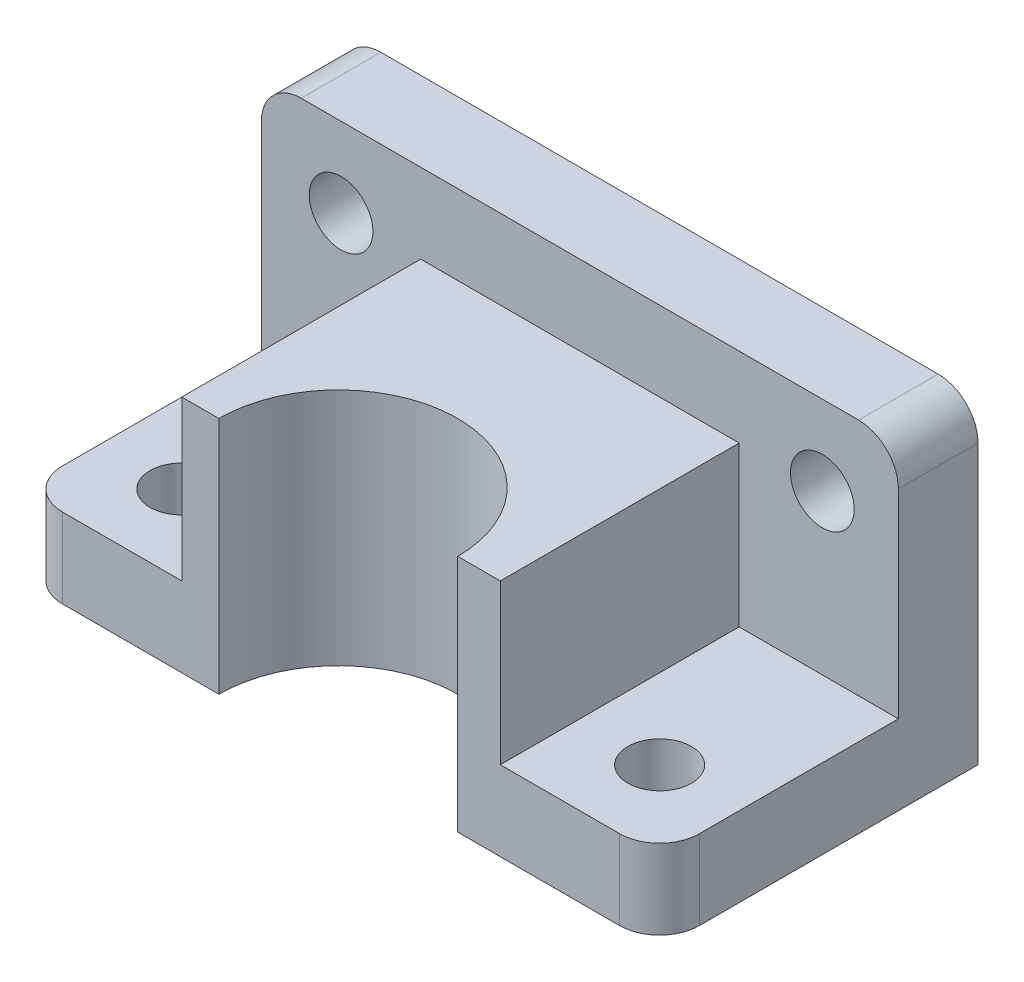
ISO-10303-21;
HEADER;
FILE_DESCRIPTION(('STEP AP214'),'2;1');
FILE_NAME('part.step','',(''),(''),'','','');
FILE_SCHEMA(('AUTOMOTIVE_DESIGN { 1 0 10303 214 1 1 1 1 }'));
ENDSEC;
DATA;
#1=APPLICATION_CONTEXT('core data for automotive mechanical design processes');
#2=APPLICATION_PROTOCOL_DEFINITION('international standard','automotive_design',2000,#1);
#3=PRODUCT_CONTEXT('',#1,'mechanical');
#4=PRODUCT('Part','Part','',(#3));
#5=PRODUCT_RELATED_PRODUCT_CATEGORY('part','',(#4));
#6=PRODUCT_DEFINITION_FORMATION('','',#4);
#7=PRODUCT_DEFINITION_CONTEXT('part definition',#1,'design');
#8=PRODUCT_DEFINITION('design','',#6,#7);
#9=PRODUCT_DEFINITION_SHAPE('','',#8);
#10=(LENGTH_UNIT() NAMED_UNIT(*) SI_UNIT(.MILLI.,.METRE.));
#11=(NAMED_UNIT(*) PLANE_ANGLE_UNIT() SI_UNIT($,.RADIAN.));
#12=(NAMED_UNIT(*) SI_UNIT($,.STERADIAN.) SOLID_ANGLE_UNIT());
#13=UNCERTAINTY_MEASURE_WITH_UNIT(LENGTH_MEASURE(1.E-05),#10,'distance_accuracy_value','');
#14=(GEOMETRIC_REPRESENTATION_CONTEXT(3) GLOBAL_UNCERTAINTY_ASSIGNED_CONTEXT((#13)) GLOBAL_UNIT_ASSIGNED_CONTEXT((#10,
#11,#12)) REPRESENTATION_CONTEXT('',''));
#15=CARTESIAN_POINT('',(0.,0.,0.));
#16=DIRECTION('',(0.,0.,1.));
#17=DIRECTION('',(1.,0.,0.));
#18=AXIS2_PLACEMENT_3D('',#15,#16,#17);
#19=CARTESIAN_POINT('',(5.,35.,10.));
#20=DIRECTION('',(0.,0.,1.));
#21=DIRECTION('',(1.,0.,0.));
#22=AXIS2_PLACEMENT_3D('',#19,#20,#21);
#23=PLANE('',#22);
#24=CARTESIAN_POINT('',(10.,30.,10.));
#25=DIRECTION('',(0.,0.,1.));
#26=DIRECTION('',(1.,0.,0.));
#27=AXIS2_PLACEMENT_3D('',#24,#25,#26);
#28=CIRCLE('',#27,4.);
#29=CARTESIAN_POINT('',(14.,30.,10.));
#30=VERTEX_POINT('',#29);
#31=EDGE_CURVE('E412',#30,#30,#28,.T.);
#32=ORIENTED_EDGE('',*,*,#31,.F.);
#33=EDGE_LOOP('',(#32));
#34=FACE_BOUND('',#33,.T.);
#35=CARTESIAN_POINT('',(70.4471624611322,30.,10.));
#36=DIRECTION('',(0.,0.,1.));
#37=DIRECTION('',(1.,0.,0.));
#38=AXIS2_PLACEMENT_3D('',#35,#36,#37);
#39=CIRCLE('',#38,3.99999999999999);
#40=CARTESIAN_POINT('',(74.4471624611322,30.,10.));
#41=VERTEX_POINT('',#40);
#42=EDGE_CURVE('E404',#41,#41,#39,.T.);
#43=ORIENTED_EDGE('',*,*,#42,.F.);
#44=EDGE_LOOP('',(#43));
#45=FACE_BOUND('',#44,.T.);
#46=DIRECTION('',(0.,-1.,0.));
#47=VECTOR('',#46,1.);
#48=CARTESIAN_POINT('',(20.,30.,10.));
#49=LINE('',#48,#47);
#50=CARTESIAN_POINT('',(20.,30.,10.));
#51=VERTEX_POINT('',#50);
#52=CARTESIAN_POINT('',(20.,10.,10.));
#53=VERTEX_POINT('',#52);
#54=EDGE_CURVE('E63',#51,#53,#49,.T.);
#55=ORIENTED_EDGE('',*,*,#54,.F.);
#56=DIRECTION('',(1.,0.,0.));
#57=VECTOR('',#56,1.);
#58=CARTESIAN_POINT('',(20.,30.,10.));
#59=LINE('',#58,#57);
#60=CARTESIAN_POINT('',(60.,30.,10.));
#61=VERTEX_POINT('',#60);
#62=EDGE_CURVE('E58',#51,#61,#59,.T.);
#63=ORIENTED_EDGE('',*,*,#62,.T.);
#64=DIRECTION('',(0.,-1.,0.));
#65=VECTOR('',#64,1.);
#66=CARTESIAN_POINT('',(60.,30.,10.));
#67=LINE('',#66,#65);
#68=CARTESIAN_POINT('',(60.,10.,10.));
#69=VERTEX_POINT('',#68);
#70=EDGE_CURVE('E171',#61,#69,#67,.T.);
#71=ORIENTED_EDGE('',*,*,#70,.T.);
#72=DIRECTION('',(1.,0.,0.));
#73=VECTOR('',#72,1.);
#74=CARTESIAN_POINT('',(60.,10.,10.));
#75=LINE('',#74,#73);
#76=CARTESIAN_POINT('',(80.,10.,10.));
#77=VERTEX_POINT('',#76);
#78=EDGE_CURVE('E206',#69,#77,#75,.T.);
#79=ORIENTED_EDGE('',*,*,#78,.T.);
#80=DIRECTION('',(0.,1.,0.));
#81=VECTOR('',#80,1.);
#82=CARTESIAN_POINT('',(80.,0.,10.));
#83=LINE('',#82,#81);
#84=CARTESIAN_POINT('',(80.,35.,10.));
#85=VERTEX_POINT('',#84);
#86=EDGE_CURVE('E259',#77,#85,#83,.T.);
#87=ORIENTED_EDGE('',*,*,#86,.T.);
#88=CARTESIAN_POINT('',(75.,35.,10.));
#89=DIRECTION('',(0.,0.,1.));
#90=DIRECTION('',(1.,0.,0.));
#91=AXIS2_PLACEMENT_3D('',#88,#89,#90);
#92=CIRCLE('',#91,5.);
#93=CARTESIAN_POINT('',(75.,40.,10.));
#94=VERTEX_POINT('',#93);
#95=EDGE_CURVE('E261',#85,#94,#92,.T.);
#96=ORIENTED_EDGE('',*,*,#95,.T.);
#97=DIRECTION('',(-1.,0.,0.));
#98=VECTOR('',#97,1.);
#99=CARTESIAN_POINT('',(5.,40.,10.));
#100=LINE('',#99,#98);
#101=CARTESIAN_POINT('',(5.,40.,10.));
#102=VERTEX_POINT('',#101);
#103=EDGE_CURVE('E263',#94,#102,#100,.T.);
#104=ORIENTED_EDGE('',*,*,#103,.T.);
#105=CARTESIAN_POINT('',(5.,35.,10.));
#106=DIRECTION('',(0.,0.,1.));
#107=DIRECTION('',(1.,0.,0.));
#108=AXIS2_PLACEMENT_3D('',#105,#106,#107);
#109=CIRCLE('',#108,5.);
#110=CARTESIAN_POINT('',(0.,35.,10.));
#111=VERTEX_POINT('',#110);
#112=EDGE_CURVE('E264',#102,#111,#109,.T.);
#113=ORIENTED_EDGE('',*,*,#112,.T.);
#114=DIRECTION('',(0.,-1.,0.));
#115=VECTOR('',#114,1.);
#116=CARTESIAN_POINT('',(0.,0.,10.));
#117=LINE('',#116,#115);
#118=CARTESIAN_POINT('',(0.,10.,10.));
#119=VERTEX_POINT('',#118);
#120=EDGE_CURVE('E253',#111,#119,#117,.T.);
#121=ORIENTED_EDGE('',*,*,#120,.T.);
#122=DIRECTION('',(1.,0.,0.));
#123=VECTOR('',#122,1.);
#124=CARTESIAN_POINT('',(0.,10.,10.));
#125=LINE('',#124,#123);
#126=EDGE_CURVE('E229',#119,#53,#125,.T.);
#127=ORIENTED_EDGE('',*,*,#126,.T.);
#128=EDGE_LOOP('',(#55,#63,#71,#79,#87,#96,#104,#113,#121,#127));
#129=FACE_BOUND('',#128,.T.);
#130=ADVANCED_FACE('F44',(#34,#45,#129),#23,.T.);
#131=CARTESIAN_POINT('',(0.,0.,10.));
#132=DIRECTION('',(1.,0.,0.));
#133=DIRECTION('',(0.,0.,-1.));
#134=AXIS2_PLACEMENT_3D('',#131,#132,#133);
#135=PLANE('',#134);
#136=DIRECTION('',(0.,-1.,0.));
#137=VECTOR('',#136,1.);
#138=CARTESIAN_POINT('',(0.,0.,0.));
#139=LINE('',#138,#137);
#140=CARTESIAN_POINT('',(0.,35.,0.));
#141=VERTEX_POINT('',#140);
#142=CARTESIAN_POINT('',(0.,0.,0.));
#143=VERTEX_POINT('',#142);
#144=EDGE_CURVE('E254',#141,#143,#139,.T.);
#145=ORIENTED_EDGE('',*,*,#144,.T.);
#146=DIRECTION('',(0.,0.,-1.));
#147=VECTOR('',#146,1.);
#148=CARTESIAN_POINT('',(0.,0.,10.));
#149=LINE('',#148,#147);
#150=CARTESIAN_POINT('',(0.,0.,35.));
#151=VERTEX_POINT('',#150);
#152=EDGE_CURVE('E11',#151,#143,#149,.T.);
#153=ORIENTED_EDGE('',*,*,#152,.F.);
#154=DIRECTION('',(0.,-1.,0.));
#155=VECTOR('',#154,1.);
#156=CARTESIAN_POINT('',(0.,10.,35.));
#157=LINE('',#156,#155);
#158=CARTESIAN_POINT('',(0.,10.,35.));
#159=VERTEX_POINT('',#158);
#160=EDGE_CURVE('E249',#159,#151,#157,.T.);
#161=ORIENTED_EDGE('',*,*,#160,.F.);
#162=DIRECTION('',(0.,0.,-1.));
#163=VECTOR('',#162,1.);
#164=CARTESIAN_POINT('',(0.,10.,10.));
#165=LINE('',#164,#163);
#166=EDGE_CURVE('E245',#159,#119,#165,.T.);
#167=ORIENTED_EDGE('',*,*,#166,.T.);
#168=ORIENTED_EDGE('',*,*,#120,.F.);
#169=DIRECTION('',(0.,0.,-1.));
#170=VECTOR('',#169,1.);
#171=CARTESIAN_POINT('',(0.,35.,10.));
#172=LINE('',#171,#170);
#173=EDGE_CURVE('E267',#111,#141,#172,.T.);
#174=ORIENTED_EDGE('',*,*,#173,.T.);
#175=EDGE_LOOP('',(#145,#153,#161,#167,#168,#174));
#176=FACE_BOUND('',#175,.T.);
#177=ADVANCED_FACE('F50',(#176),#135,.F.);
#178=CARTESIAN_POINT('',(0.,0.,10.));
#179=DIRECTION('',(0.,1.,0.));
#180=DIRECTION('',(0.,0.,1.));
#181=AXIS2_PLACEMENT_3D('',#178,#179,#180);
#182=PLANE('',#181);
#183=CARTESIAN_POINT('',(10.,0.,30.));
#184=DIRECTION('',(0.,1.,0.));
#185=DIRECTION('',(0.,0.,1.));
#186=AXIS2_PLACEMENT_3D('',#183,#184,#185);
#187=CIRCLE('',#186,4.);
#188=CARTESIAN_POINT('',(10.,0.,34.));
#189=VERTEX_POINT('',#188);
#190=EDGE_CURVE('E399',#189,#189,#187,.T.);
#191=ORIENTED_EDGE('',*,*,#190,.T.);
#192=EDGE_LOOP('',(#191));
#193=FACE_BOUND('',#192,.T.);
#194=CARTESIAN_POINT('',(70.0171177936021,0.,30.));
#195=DIRECTION('',(0.,1.,0.));
#196=DIRECTION('',(0.,0.,1.));
#197=AXIS2_PLACEMENT_3D('',#194,#195,#196);
#198=CIRCLE('',#197,3.99999999999999);
#199=CARTESIAN_POINT('',(70.0171177936021,0.,34.));
#200=VERTEX_POINT('',#199);
#201=EDGE_CURVE('E405',#200,#200,#198,.T.);
#202=ORIENTED_EDGE('',*,*,#201,.T.);
#203=EDGE_LOOP('',(#202));
#204=FACE_BOUND('',#203,.T.);
#205=CARTESIAN_POINT('',(39.6559642659759,0.,40.));
#206=DIRECTION('',(0.,1.,0.));
#207=DIRECTION('',(0.,0.,-1.));
#208=AXIS2_PLACEMENT_3D('',#205,#206,#207);
#209=CIRCLE('',#208,15.);
#210=CARTESIAN_POINT('',(54.6559642659759,0.,40.));
#211=VERTEX_POINT('',#210);
#212=CARTESIAN_POINT('',(24.6559642659759,0.,40.));
#213=VERTEX_POINT('',#212);
#214=EDGE_CURVE('E183',#211,#213,#209,.T.);
#215=ORIENTED_EDGE('',*,*,#214,.T.);
#216=DIRECTION('',(-1.,0.,0.));
#217=VECTOR('',#216,1.);
#218=CARTESIAN_POINT('',(5.,0.,40.));
#219=LINE('',#218,#217);
#220=CARTESIAN_POINT('',(5.,0.,40.));
#221=VERTEX_POINT('',#220);
#222=EDGE_CURVE('E227',#213,#221,#219,.T.);
#223=ORIENTED_EDGE('',*,*,#222,.T.);
#224=CARTESIAN_POINT('',(5.,0.,35.));
#225=DIRECTION('',(0.,-1.,0.));
#226=DIRECTION('',(0.,0.,-1.));
#227=AXIS2_PLACEMENT_3D('',#224,#225,#226);
#228=CIRCLE('',#227,5.);
#229=EDGE_CURVE('E231',#221,#151,#228,.T.);
#230=ORIENTED_EDGE('',*,*,#229,.T.);
#231=ORIENTED_EDGE('',*,*,#152,.T.);
#232=DIRECTION('',(1.,0.,0.));
#233=VECTOR('',#232,1.);
#234=CARTESIAN_POINT('',(0.,0.,0.));
#235=LINE('',#234,#233);
#236=CARTESIAN_POINT('',(80.,0.,0.));
#237=VERTEX_POINT('',#236);
#238=EDGE_CURVE('E270',#143,#237,#235,.T.);
#239=ORIENTED_EDGE('',*,*,#238,.T.);
#240=DIRECTION('',(0.,0.,-1.));
#241=VECTOR('',#240,1.);
#242=CARTESIAN_POINT('',(80.,0.,10.));
#243=LINE('',#242,#241);
#244=CARTESIAN_POINT('',(80.,0.,35.));
#245=VERTEX_POINT('',#244);
#246=EDGE_CURVE('E52',#245,#237,#243,.T.);
#247=ORIENTED_EDGE('',*,*,#246,.F.);
#248=CARTESIAN_POINT('',(75.,0.,35.));
#249=DIRECTION('',(0.,-1.,0.));
#250=DIRECTION('',(0.,0.,-1.));
#251=AXIS2_PLACEMENT_3D('',#248,#249,#250);
#252=CIRCLE('',#251,5.);
#253=CARTESIAN_POINT('',(75.,0.,40.));
#254=VERTEX_POINT('',#253);
#255=EDGE_CURVE('E197',#245,#254,#252,.T.);
#256=ORIENTED_EDGE('',*,*,#255,.T.);
#257=DIRECTION('',(-1.,0.,0.));
#258=VECTOR('',#257,1.);
#259=CARTESIAN_POINT('',(60.,0.,40.));
#260=LINE('',#259,#258);
#261=EDGE_CURVE('E215',#254,#211,#260,.T.);
#262=ORIENTED_EDGE('',*,*,#261,.T.);
#263=EDGE_LOOP('',(#215,#223,#230,#231,#239,#247,#256,#262));
#264=FACE_BOUND('',#263,.T.);
#265=ADVANCED_FACE('F319',(#193,#204,#264),#182,.F.);
#266=CARTESIAN_POINT('',(80.,0.,10.));
#267=DIRECTION('',(-1.,0.,0.));
#268=DIRECTION('',(0.,0.,1.));
#269=AXIS2_PLACEMENT_3D('',#266,#267,#268);
#270=PLANE('',#269);
#271=DIRECTION('',(0.,1.,0.));
#272=VECTOR('',#271,1.);
#273=CARTESIAN_POINT('',(80.,0.,0.));
#274=LINE('',#273,#272);
#275=CARTESIAN_POINT('',(80.,35.,0.));
#276=VERTEX_POINT('',#275);
#277=EDGE_CURVE('E275',#237,#276,#274,.T.);
#278=ORIENTED_EDGE('',*,*,#277,.T.);
#279=DIRECTION('',(0.,0.,-1.));
#280=VECTOR('',#279,1.);
#281=CARTESIAN_POINT('',(80.,35.,10.));
#282=LINE('',#281,#280);
#283=EDGE_CURVE('E287',#85,#276,#282,.T.);
#284=ORIENTED_EDGE('',*,*,#283,.F.);
#285=ORIENTED_EDGE('',*,*,#86,.F.);
#286=DIRECTION('',(0.,0.,1.));
#287=VECTOR('',#286,1.);
#288=CARTESIAN_POINT('',(80.,10.,10.));
#289=LINE('',#288,#287);
#290=CARTESIAN_POINT('',(80.,10.,35.));
#291=VERTEX_POINT('',#290);
#292=EDGE_CURVE('E212',#77,#291,#289,.T.);
#293=ORIENTED_EDGE('',*,*,#292,.T.);
#294=DIRECTION('',(0.,-1.,0.));
#295=VECTOR('',#294,1.);
#296=CARTESIAN_POINT('',(80.,10.,35.));
#297=LINE('',#296,#295);
#298=EDGE_CURVE('E221',#291,#245,#297,.T.);
#299=ORIENTED_EDGE('',*,*,#298,.T.);
#300=ORIENTED_EDGE('',*,*,#246,.T.);
#301=EDGE_LOOP('',(#278,#284,#285,#293,#299,#300));
#302=FACE_BOUND('',#301,.T.);
#303=ADVANCED_FACE('F292',(#302),#270,.F.);
#304=CARTESIAN_POINT('',(75.,35.,10.));
#305=DIRECTION('',(0.,0.,-1.));
#306=DIRECTION('',(-1.,0.,0.));
#307=AXIS2_PLACEMENT_3D('',#304,#305,#306);
#308=CYLINDRICAL_SURFACE('',#307,5.);
#309=CARTESIAN_POINT('',(75.,35.,0.));
#310=DIRECTION('',(0.,0.,1.));
#311=DIRECTION('',(1.,0.,0.));
#312=AXIS2_PLACEMENT_3D('',#309,#310,#311);
#313=CIRCLE('',#312,5.);
#314=CARTESIAN_POINT('',(75.,40.,0.));
#315=VERTEX_POINT('',#314);
#316=EDGE_CURVE('E274',#276,#315,#313,.T.);
#317=ORIENTED_EDGE('',*,*,#316,.T.);
#318=DIRECTION('',(0.,0.,-1.));
#319=VECTOR('',#318,1.);
#320=CARTESIAN_POINT('',(75.,40.,10.));
#321=LINE('',#320,#319);
#322=EDGE_CURVE('E282',#94,#315,#321,.T.);
#323=ORIENTED_EDGE('',*,*,#322,.F.);
#324=ORIENTED_EDGE('',*,*,#95,.F.);
#325=ORIENTED_EDGE('',*,*,#283,.T.);
#326=EDGE_LOOP('',(#317,#323,#324,#325));
#327=FACE_BOUND('',#326,.T.);
#328=ADVANCED_FACE('F302',(#327),#308,.T.);
#329=CARTESIAN_POINT('',(5.,40.,10.));
#330=DIRECTION('',(0.,-1.,0.));
#331=DIRECTION('',(1.,0.,0.));
#332=AXIS2_PLACEMENT_3D('',#329,#330,#331);
#333=PLANE('',#332);
#334=DIRECTION('',(-1.,0.,0.));
#335=VECTOR('',#334,1.);
#336=CARTESIAN_POINT('',(5.,40.,0.));
#337=LINE('',#336,#335);
#338=CARTESIAN_POINT('',(5.,40.,0.));
#339=VERTEX_POINT('',#338);
#340=EDGE_CURVE('E277',#315,#339,#337,.T.);
#341=ORIENTED_EDGE('',*,*,#340,.T.);
#342=DIRECTION('',(0.,0.,-1.));
#343=VECTOR('',#342,1.);
#344=CARTESIAN_POINT('',(5.,40.,10.));
#345=LINE('',#344,#343);
#346=EDGE_CURVE('E281',#102,#339,#345,.T.);
#347=ORIENTED_EDGE('',*,*,#346,.F.);
#348=ORIENTED_EDGE('',*,*,#103,.F.);
#349=ORIENTED_EDGE('',*,*,#322,.T.);
#350=EDGE_LOOP('',(#341,#347,#348,#349));
#351=FACE_BOUND('',#350,.T.);
#352=ADVANCED_FACE('F308',(#351),#333,.F.);
#353=CARTESIAN_POINT('',(5.,35.,10.));
#354=DIRECTION('',(0.,0.,-1.));
#355=DIRECTION('',(-1.,0.,0.));
#356=AXIS2_PLACEMENT_3D('',#353,#354,#355);
#357=CYLINDRICAL_SURFACE('',#356,5.);
#358=CARTESIAN_POINT('',(5.,35.,0.));
#359=DIRECTION('',(0.,0.,1.));
#360=DIRECTION('',(1.,0.,0.));
#361=AXIS2_PLACEMENT_3D('',#358,#359,#360);
#362=CIRCLE('',#361,5.);
#363=EDGE_CURVE('E256',#339,#141,#362,.T.);
#364=ORIENTED_EDGE('',*,*,#363,.T.);
#365=ORIENTED_EDGE('',*,*,#173,.F.);
#366=ORIENTED_EDGE('',*,*,#112,.F.);
#367=ORIENTED_EDGE('',*,*,#346,.T.);
#368=EDGE_LOOP('',(#364,#365,#366,#367));
#369=FACE_BOUND('',#368,.T.);
#370=ADVANCED_FACE('F340',(#369),#357,.T.);
#371=CARTESIAN_POINT('',(5.,35.,0.));
#372=DIRECTION('',(0.,0.,1.));
#373=DIRECTION('',(1.,0.,0.));
#374=AXIS2_PLACEMENT_3D('',#371,#372,#373);
#375=PLANE('',#374);
#376=CARTESIAN_POINT('',(10.,30.,0.));
#377=DIRECTION('',(0.,0.,1.));
#378=DIRECTION('',(1.,0.,0.));
#379=AXIS2_PLACEMENT_3D('',#376,#377,#378);
#380=CIRCLE('',#379,4.);
#381=CARTESIAN_POINT('',(14.,30.,0.));
#382=VERTEX_POINT('',#381);
#383=EDGE_CURVE('E200',#382,#382,#380,.T.);
#384=ORIENTED_EDGE('',*,*,#383,.T.);
#385=EDGE_LOOP('',(#384));
#386=FACE_BOUND('',#385,.T.);
#387=CARTESIAN_POINT('',(70.4471624611322,30.,0.));
#388=DIRECTION('',(0.,0.,1.));
#389=DIRECTION('',(1.,0.,0.));
#390=AXIS2_PLACEMENT_3D('',#387,#388,#389);
#391=CIRCLE('',#390,3.99999999999999);
#392=CARTESIAN_POINT('',(74.4471624611322,30.,0.));
#393=VERTEX_POINT('',#392);
#394=EDGE_CURVE('E417',#393,#393,#391,.T.);
#395=ORIENTED_EDGE('',*,*,#394,.T.);
#396=EDGE_LOOP('',(#395));
#397=FACE_BOUND('',#396,.T.);
#398=ORIENTED_EDGE('',*,*,#144,.F.);
#399=ORIENTED_EDGE('',*,*,#363,.F.);
#400=ORIENTED_EDGE('',*,*,#340,.F.);
#401=ORIENTED_EDGE('',*,*,#316,.F.);
#402=ORIENTED_EDGE('',*,*,#277,.F.);
#403=ORIENTED_EDGE('',*,*,#238,.F.);
#404=EDGE_LOOP('',(#398,#399,#400,#401,#402,#403));
#405=FACE_BOUND('',#404,.T.);
#406=ADVANCED_FACE('F299',(#386,#397,#405),#375,.F.);
#407=CARTESIAN_POINT('',(5.,10.,35.));
#408=DIRECTION('',(0.,-1.,0.));
#409=DIRECTION('',(0.,0.,-1.));
#410=AXIS2_PLACEMENT_3D('',#407,#408,#409);
#411=CYLINDRICAL_SURFACE('',#410,5.);
#412=ORIENTED_EDGE('',*,*,#229,.F.);
#413=DIRECTION('',(0.,-1.,0.));
#414=VECTOR('',#413,1.);
#415=CARTESIAN_POINT('',(5.,10.,40.));
#416=LINE('',#415,#414);
#417=CARTESIAN_POINT('',(5.,10.,40.));
#418=VERTEX_POINT('',#417);
#419=EDGE_CURVE('E244',#418,#221,#416,.T.);
#420=ORIENTED_EDGE('',*,*,#419,.F.);
#421=CARTESIAN_POINT('',(5.,10.,35.));
#422=DIRECTION('',(0.,-1.,0.));
#423=DIRECTION('',(0.,0.,-1.));
#424=AXIS2_PLACEMENT_3D('',#421,#422,#423);
#425=CIRCLE('',#424,5.);
#426=EDGE_CURVE('E237',#418,#159,#425,.T.);
#427=ORIENTED_EDGE('',*,*,#426,.T.);
#428=ORIENTED_EDGE('',*,*,#160,.T.);
#429=EDGE_LOOP('',(#412,#420,#427,#428));
#430=FACE_BOUND('',#429,.T.);
#431=ADVANCED_FACE('F334',(#430),#411,.T.);
#432=CARTESIAN_POINT('',(5.,10.,40.));
#433=DIRECTION('',(0.,0.,1.));
#434=DIRECTION('',(1.,0.,0.));
#435=AXIS2_PLACEMENT_3D('',#432,#433,#434);
#436=PLANE('',#435);
#437=ORIENTED_EDGE('',*,*,#222,.F.);
#438=DIRECTION('',(0.,-1.,0.));
#439=VECTOR('',#438,1.);
#440=CARTESIAN_POINT('',(24.6559642659759,30.,40.));
#441=LINE('',#440,#439);
#442=CARTESIAN_POINT('',(24.6559642659759,30.,40.));
#443=VERTEX_POINT('',#442);
#444=EDGE_CURVE('E204',#443,#213,#441,.T.);
#445=ORIENTED_EDGE('',*,*,#444,.F.);
#446=DIRECTION('',(-1.,0.,0.));
#447=VECTOR('',#446,1.);
#448=CARTESIAN_POINT('',(20.,30.,40.));
#449=LINE('',#448,#447);
#450=CARTESIAN_POINT('',(20.,30.,40.));
#451=VERTEX_POINT('',#450);
#452=EDGE_CURVE('E186',#443,#451,#449,.T.);
#453=ORIENTED_EDGE('',*,*,#452,.T.);
#454=DIRECTION('',(0.,-1.,0.));
#455=VECTOR('',#454,1.);
#456=CARTESIAN_POINT('',(20.,30.,40.));
#457=LINE('',#456,#455);
#458=CARTESIAN_POINT('',(20.,10.,40.));
#459=VERTEX_POINT('',#458);
#460=EDGE_CURVE('E199',#451,#459,#457,.T.);
#461=ORIENTED_EDGE('',*,*,#460,.T.);
#462=DIRECTION('',(-1.,0.,0.));
#463=VECTOR('',#462,1.);
#464=CARTESIAN_POINT('',(5.,10.,40.));
#465=LINE('',#464,#463);
#466=EDGE_CURVE('E236',#459,#418,#465,.T.);
#467=ORIENTED_EDGE('',*,*,#466,.T.);
#468=ORIENTED_EDGE('',*,*,#419,.T.);
#469=EDGE_LOOP('',(#437,#445,#453,#461,#467,#468));
#470=FACE_BOUND('',#469,.T.);
#471=ADVANCED_FACE('F324',(#470),#436,.T.);
#472=CARTESIAN_POINT('',(5.,10.,35.));
#473=DIRECTION('',(0.,-1.,0.));
#474=DIRECTION('',(0.,0.,-1.));
#475=AXIS2_PLACEMENT_3D('',#472,#473,#474);
#476=PLANE('',#475);
#477=CARTESIAN_POINT('',(10.,10.,30.));
#478=DIRECTION('',(0.,1.,0.));
#479=DIRECTION('',(0.,0.,1.));
#480=AXIS2_PLACEMENT_3D('',#477,#478,#479);
#481=CIRCLE('',#480,4.);
#482=CARTESIAN_POINT('',(10.,10.,34.));
#483=VERTEX_POINT('',#482);
#484=EDGE_CURVE('E402',#483,#483,#481,.T.);
#485=ORIENTED_EDGE('',*,*,#484,.F.);
#486=EDGE_LOOP('',(#485));
#487=FACE_BOUND('',#486,.T.);
#488=ORIENTED_EDGE('',*,*,#126,.F.);
#489=ORIENTED_EDGE('',*,*,#166,.F.);
#490=ORIENTED_EDGE('',*,*,#426,.F.);
#491=ORIENTED_EDGE('',*,*,#466,.F.);
#492=DIRECTION('',(0.,0.,1.));
#493=VECTOR('',#492,1.);
#494=CARTESIAN_POINT('',(20.,10.,10.));
#495=LINE('',#494,#493);
#496=EDGE_CURVE('E235',#53,#459,#495,.T.);
#497=ORIENTED_EDGE('',*,*,#496,.F.);
#498=EDGE_LOOP('',(#488,#489,#490,#491,#497));
#499=FACE_BOUND('',#498,.T.);
#500=ADVANCED_FACE('F329',(#487,#499),#476,.F.);
#501=CARTESIAN_POINT('',(60.,10.,40.));
#502=DIRECTION('',(0.,0.,1.));
#503=DIRECTION('',(1.,0.,0.));
#504=AXIS2_PLACEMENT_3D('',#501,#502,#503);
#505=PLANE('',#504);
#506=ORIENTED_EDGE('',*,*,#261,.F.);
#507=DIRECTION('',(0.,-1.,0.));
#508=VECTOR('',#507,1.);
#509=CARTESIAN_POINT('',(75.,10.,40.));
#510=LINE('',#509,#508);
#511=CARTESIAN_POINT('',(75.,10.,40.));
#512=VERTEX_POINT('',#511);
#513=EDGE_CURVE('E225',#512,#254,#510,.T.);
#514=ORIENTED_EDGE('',*,*,#513,.F.);
#515=DIRECTION('',(-1.,0.,0.));
#516=VECTOR('',#515,1.);
#517=CARTESIAN_POINT('',(60.,10.,40.));
#518=LINE('',#517,#516);
#519=CARTESIAN_POINT('',(60.,10.,40.));
#520=VERTEX_POINT('',#519);
#521=EDGE_CURVE('E164',#512,#520,#518,.T.);
#522=ORIENTED_EDGE('',*,*,#521,.T.);
#523=DIRECTION('',(0.,-1.,0.));
#524=VECTOR('',#523,1.);
#525=CARTESIAN_POINT('',(60.,30.,40.));
#526=LINE('',#525,#524);
#527=CARTESIAN_POINT('',(60.,30.,40.));
#528=VERTEX_POINT('',#527);
#529=EDGE_CURVE('E159',#528,#520,#526,.T.);
#530=ORIENTED_EDGE('',*,*,#529,.F.);
#531=DIRECTION('',(-1.,0.,0.));
#532=VECTOR('',#531,1.);
#533=CARTESIAN_POINT('',(60.,30.,40.));
#534=LINE('',#533,#532);
#535=CARTESIAN_POINT('',(54.6559642659759,30.,40.));
#536=VERTEX_POINT('',#535);
#537=EDGE_CURVE('E161',#528,#536,#534,.T.);
#538=ORIENTED_EDGE('',*,*,#537,.T.);
#539=DIRECTION('',(0.,-1.,0.));
#540=VECTOR('',#539,1.);
#541=CARTESIAN_POINT('',(54.6559642659759,30.,40.));
#542=LINE('',#541,#540);
#543=EDGE_CURVE('E167',#536,#211,#542,.T.);
#544=ORIENTED_EDGE('',*,*,#543,.T.);
#545=EDGE_LOOP('',(#506,#514,#522,#530,#538,#544));
#546=FACE_BOUND('',#545,.T.);
#547=ADVANCED_FACE('F163',(#546),#505,.T.);
#548=CARTESIAN_POINT('',(75.,10.,35.));
#549=DIRECTION('',(0.,-1.,0.));
#550=DIRECTION('',(0.,0.,-1.));
#551=AXIS2_PLACEMENT_3D('',#548,#549,#550);
#552=CYLINDRICAL_SURFACE('',#551,5.);
#553=ORIENTED_EDGE('',*,*,#255,.F.);
#554=ORIENTED_EDGE('',*,*,#298,.F.);
#555=CARTESIAN_POINT('',(75.,10.,35.));
#556=DIRECTION('',(0.,-1.,0.));
#557=DIRECTION('',(0.,0.,-1.));
#558=AXIS2_PLACEMENT_3D('',#555,#556,#557);
#559=CIRCLE('',#558,5.);
#560=EDGE_CURVE('E213',#291,#512,#559,.T.);
#561=ORIENTED_EDGE('',*,*,#560,.T.);
#562=ORIENTED_EDGE('',*,*,#513,.T.);
#563=EDGE_LOOP('',(#553,#554,#561,#562));
#564=FACE_BOUND('',#563,.T.);
#565=ADVANCED_FACE('F320',(#564),#552,.T.);
#566=CARTESIAN_POINT('',(75.,10.,35.));
#567=DIRECTION('',(0.,-1.,0.));
#568=DIRECTION('',(0.,0.,-1.));
#569=AXIS2_PLACEMENT_3D('',#566,#567,#568);
#570=PLANE('',#569);
#571=CARTESIAN_POINT('',(70.0171177936021,10.,30.));
#572=DIRECTION('',(0.,1.,0.));
#573=DIRECTION('',(0.,0.,1.));
#574=AXIS2_PLACEMENT_3D('',#571,#572,#573);
#575=CIRCLE('',#574,3.99999999999999);
#576=CARTESIAN_POINT('',(70.0171177936021,10.,34.));
#577=VERTEX_POINT('',#576);
#578=EDGE_CURVE('E410',#577,#577,#575,.T.);
#579=ORIENTED_EDGE('',*,*,#578,.F.);
#580=EDGE_LOOP('',(#579));
#581=FACE_BOUND('',#580,.T.);
#582=ORIENTED_EDGE('',*,*,#78,.F.);
#583=DIRECTION('',(0.,0.,-1.));
#584=VECTOR('',#583,1.);
#585=CARTESIAN_POINT('',(60.,10.,10.));
#586=LINE('',#585,#584);
#587=EDGE_CURVE('E217',#520,#69,#586,.T.);
#588=ORIENTED_EDGE('',*,*,#587,.F.);
#589=ORIENTED_EDGE('',*,*,#521,.F.);
#590=ORIENTED_EDGE('',*,*,#560,.F.);
#591=ORIENTED_EDGE('',*,*,#292,.F.);
#592=EDGE_LOOP('',(#582,#588,#589,#590,#591));
#593=FACE_BOUND('',#592,.T.);
#594=ADVANCED_FACE('F314',(#581,#593),#570,.F.);
#595=CARTESIAN_POINT('',(20.,30.,10.));
#596=DIRECTION('',(-1.,0.,0.));
#597=DIRECTION('',(0.,0.,1.));
#598=AXIS2_PLACEMENT_3D('',#595,#596,#597);
#599=PLANE('',#598);
#600=ORIENTED_EDGE('',*,*,#496,.T.);
#601=ORIENTED_EDGE('',*,*,#460,.F.);
#602=DIRECTION('',(0.,0.,-1.));
#603=VECTOR('',#602,1.);
#604=CARTESIAN_POINT('',(20.,30.,10.));
#605=LINE('',#604,#603);
#606=EDGE_CURVE('E195',#451,#51,#605,.T.);
#607=ORIENTED_EDGE('',*,*,#606,.T.);
#608=ORIENTED_EDGE('',*,*,#54,.T.);
#609=EDGE_LOOP('',(#600,#601,#607,#608));
#610=FACE_BOUND('',#609,.T.);
#611=ADVANCED_FACE('F326',(#610),#599,.T.);
#612=CARTESIAN_POINT('',(60.,30.,10.));
#613=DIRECTION('',(1.,0.,0.));
#614=DIRECTION('',(0.,0.,-1.));
#615=AXIS2_PLACEMENT_3D('',#612,#613,#614);
#616=PLANE('',#615);
#617=ORIENTED_EDGE('',*,*,#587,.T.);
#618=ORIENTED_EDGE('',*,*,#70,.F.);
#619=DIRECTION('',(0.,0.,1.));
#620=VECTOR('',#619,1.);
#621=CARTESIAN_POINT('',(60.,30.,10.));
#622=LINE('',#621,#620);
#623=EDGE_CURVE('E180',#61,#528,#622,.T.);
#624=ORIENTED_EDGE('',*,*,#623,.T.);
#625=ORIENTED_EDGE('',*,*,#529,.T.);
#626=EDGE_LOOP('',(#617,#618,#624,#625));
#627=FACE_BOUND('',#626,.T.);
#628=ADVANCED_FACE('F185',(#627),#616,.T.);
#629=CARTESIAN_POINT('',(39.6559642659759,30.,40.));
#630=DIRECTION('',(0.,-1.,0.));
#631=DIRECTION('',(0.,0.,-1.));
#632=AXIS2_PLACEMENT_3D('',#629,#630,#631);
#633=CYLINDRICAL_SURFACE('',#632,15.);
#634=ORIENTED_EDGE('',*,*,#214,.F.);
#635=ORIENTED_EDGE('',*,*,#543,.F.);
#636=CARTESIAN_POINT('',(39.6559642659759,30.,40.));
#637=DIRECTION('',(0.,1.,0.));
#638=DIRECTION('',(0.,0.,-1.));
#639=AXIS2_PLACEMENT_3D('',#636,#637,#638);
#640=CIRCLE('',#639,15.);
#641=EDGE_CURVE('E179',#536,#443,#640,.T.);
#642=ORIENTED_EDGE('',*,*,#641,.T.);
#643=ORIENTED_EDGE('',*,*,#444,.T.);
#644=EDGE_LOOP('',(#634,#635,#642,#643));
#645=FACE_BOUND('',#644,.T.);
#646=ADVANCED_FACE('F322',(#645),#633,.F.);
#647=CARTESIAN_POINT('',(39.6559642659759,30.,40.));
#648=DIRECTION('',(0.,-1.,0.));
#649=DIRECTION('',(0.,0.,-1.));
#650=AXIS2_PLACEMENT_3D('',#647,#648,#649);
#651=PLANE('',#650);
#652=ORIENTED_EDGE('',*,*,#62,.F.);
#653=ORIENTED_EDGE('',*,*,#606,.F.);
#654=ORIENTED_EDGE('',*,*,#452,.F.);
#655=ORIENTED_EDGE('',*,*,#641,.F.);
#656=ORIENTED_EDGE('',*,*,#537,.F.);
#657=ORIENTED_EDGE('',*,*,#623,.F.);
#658=EDGE_LOOP('',(#652,#653,#654,#655,#656,#657));
#659=FACE_BOUND('',#658,.T.);
#660=ADVANCED_FACE('F176',(#659),#651,.F.);
#661=CARTESIAN_POINT('',(70.4471624611322,30.,0.));
#662=DIRECTION('',(0.,0.,1.));
#663=DIRECTION('',(1.,0.,0.));
#664=AXIS2_PLACEMENT_3D('',#661,#662,#663);
#665=CYLINDRICAL_SURFACE('',#664,3.99999999999999);
#666=ORIENTED_EDGE('',*,*,#394,.F.);
#667=EDGE_LOOP('',(#666));
#668=FACE_BOUND('',#667,.T.);
#669=ORIENTED_EDGE('',*,*,#42,.T.);
#670=EDGE_LOOP('',(#669));
#671=FACE_BOUND('',#670,.T.);
#672=ADVANCED_FACE('F377',(#668,#671),#665,.F.);
#673=CARTESIAN_POINT('',(10.,30.,0.));
#674=DIRECTION('',(0.,0.,1.));
#675=DIRECTION('',(1.,0.,0.));
#676=AXIS2_PLACEMENT_3D('',#673,#674,#675);
#677=CYLINDRICAL_SURFACE('',#676,4.);
#678=ORIENTED_EDGE('',*,*,#383,.F.);
#679=EDGE_LOOP('',(#678));
#680=FACE_BOUND('',#679,.T.);
#681=ORIENTED_EDGE('',*,*,#31,.T.);
#682=EDGE_LOOP('',(#681));
#683=FACE_BOUND('',#682,.T.);
#684=ADVANCED_FACE('F382',(#680,#683),#677,.F.);
#685=CARTESIAN_POINT('',(70.0171177936021,0.,30.));
#686=DIRECTION('',(0.,1.,0.));
#687=DIRECTION('',(0.,0.,1.));
#688=AXIS2_PLACEMENT_3D('',#685,#686,#687);
#689=CYLINDRICAL_SURFACE('',#688,3.99999999999999);
#690=ORIENTED_EDGE('',*,*,#201,.F.);
#691=EDGE_LOOP('',(#690));
#692=FACE_BOUND('',#691,.T.);
#693=ORIENTED_EDGE('',*,*,#578,.T.);
#694=EDGE_LOOP('',(#693));
#695=FACE_BOUND('',#694,.T.);
#696=ADVANCED_FACE('F383',(#692,#695),#689,.F.);
#697=CARTESIAN_POINT('',(10.,0.,30.));
#698=DIRECTION('',(0.,1.,0.));
#699=DIRECTION('',(0.,0.,1.));
#700=AXIS2_PLACEMENT_3D('',#697,#698,#699);
#701=CYLINDRICAL_SURFACE('',#700,4.);
#702=ORIENTED_EDGE('',*,*,#190,.F.);
#703=EDGE_LOOP('',(#702));
#704=FACE_BOUND('',#703,.T.);
#705=ORIENTED_EDGE('',*,*,#484,.T.);
#706=EDGE_LOOP('',(#705));
#707=FACE_BOUND('',#706,.T.);
#708=ADVANCED_FACE('F386',(#704,#707),#701,.F.);
#709=CLOSED_SHELL('',(#130,#177,#265,#303,#328,#352,#370,#406,#431,#471,#500,#547,#565,#594,
#611,#628,#646,#660,#672,#684,#696,#708));
#710=MANIFOLD_SOLID_BREP('B2',#709);
#711=ADVANCED_BREP_SHAPE_REPRESENTATION('',(#18,#710),#14);
#712=SHAPE_DEFINITION_REPRESENTATION(#9,#711);
ENDSEC;
END-ISO-10303-21;
